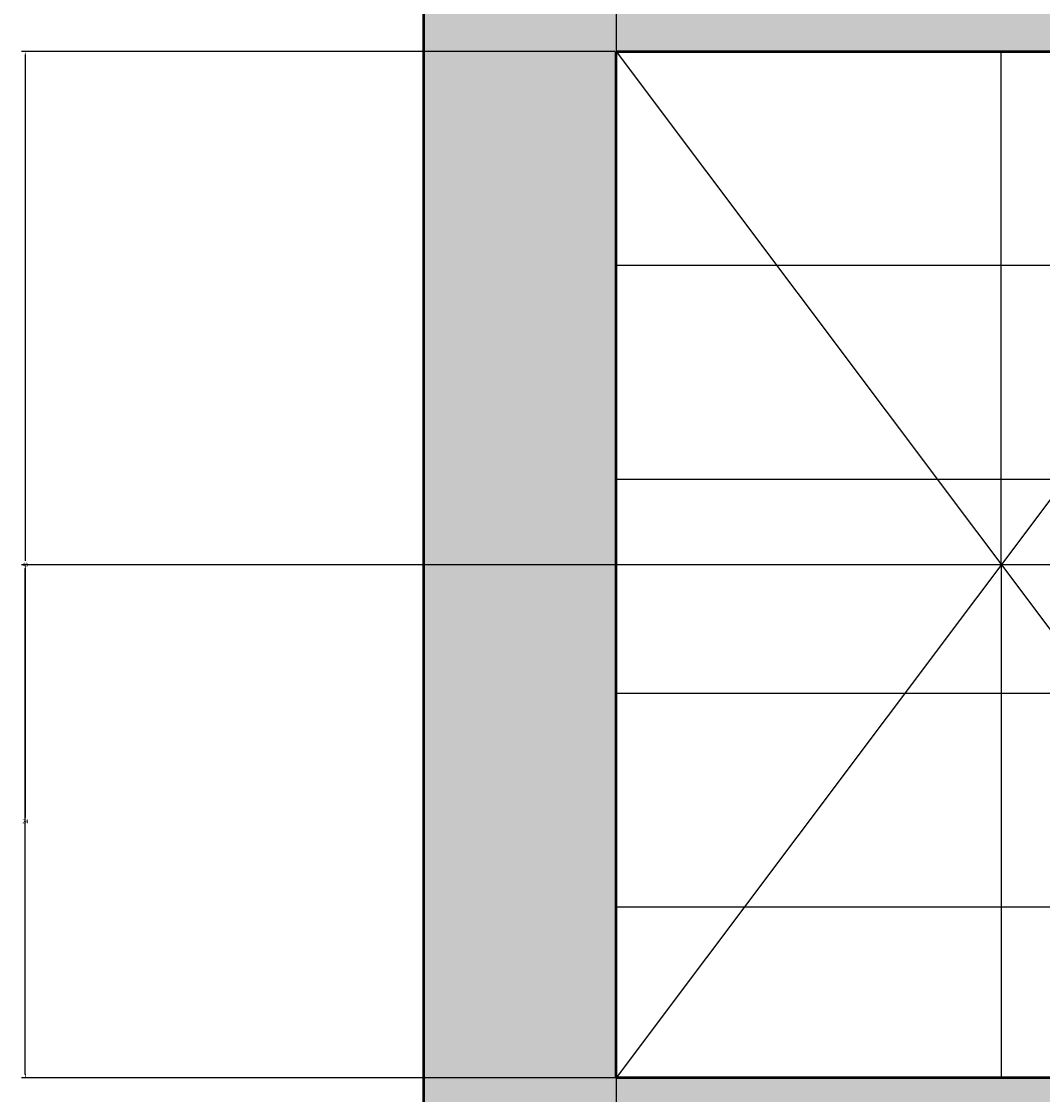
# Model space of a CAD drawing. Units: inches. Extents: x 2231 to 2461, y 2045 to 2455.
# Tile 2 of 95: x 2231 to 2279, y 2072 to 2122. Entities that reach past the tile are written whole.
import ezdxf

# ---------------------------------------------------------------- set-up
doc = ezdxf.new("R2010")
doc.units = ezdxf.units.IN
for name, color, linetype, lineweight in [('A-ANNO-DIMS', 2, 'Continuous', 18), ('A-FLOR-EVTR', 8, 'Continuous', 25), ('A-WALL', 7, 'Continuous', 50)]:
    doc.layers.add(name, color=color, linetype=linetype, lineweight=lineweight)
doc.layers.add('A-WALL-PATT', color=18, linetype='Continuous', lineweight=13, true_color=0x000000)
doc.styles.get("Standard").update_dxf_attribs({"font": 'arial.ttf'})
doc.dimstyles.get("Standard").update_dxf_attribs({"dimtxt": 0.18, "dimasz": 0.18, "dimexe": 0.18, "dimexo": 0.0625, "dimgap": 0.09, "dimtad": 0, "dimtih": 1, "dimtoh": 1, "dimdec": 4, "dimzin": 0, "dimdsep": 46, "dimtxsty": 'Standard', "dimcen": 0.09, "dimadec": 0, "dimazin": 0, "dimtfac": 1, "dimtdec": 4, "dimtofl": 0, "dimtmove": 0, "dimatfit": 3, "dimfxl": 1, "dimtolj": 1, "dimtzin": 0, "dimarcsym": 0})

# ---------------------------------------------------------------- blocks, each defined once
blk = doc.blocks.new('*D51')
at = {"layer": 'A-ANNO-DIMS', "color": 0, "lineweight": -2, "transparency": 16777216}
for p, q in [((2258.794, 2306.77), (2258.794, 2044.803)), ((2330.794, 2306.77), (2330.794, 2044.803)), ((2258.974, 2044.983), (2294.576, 2044.983)), ((2330.614, 2044.983), (2295.011, 2044.983))]:
    blk.add_line(p, q, dxfattribs=at)
at = {"layer": 'A-ANNO-DIMS', "color": 0, "transparency": 16777216}
for points in [[(2258.974, 2045.013), (2258.974, 2044.953), (2258.794, 2044.983)], [(2330.614, 2045.013), (2330.614, 2044.953), (2330.794, 2044.983)]]:
    blk.add_solid(points, dxfattribs=at)
at = {"layer": 'Defpoints', "color": 0, "transparency": 16777216}
for p in [(2258.794, 2306.833), (2330.794, 2306.833), (2330.794, 2044.983)]:
    blk.add_point(p, dxfattribs=at)
at = {"layer": 'A-ANNO-DIMS', "color": 0, "transparency": 16777216, "insert": (2294.794, 2044.983), "char_height": 0.18, "attachment_point": 5}
blk.add_mtext('\\A1;72', dxfattribs=at)
blk = doc.blocks.new('*D61')
at = {"layer": 'A-ANNO-DIMS', "color": 0, "lineweight": -2, "transparency": 16777216}
for p, q in [((2258.731, 2120.833), (2230.981, 2120.833)), ((2231.161, 2120.653), (2231.161, 2097.015)), ((2231.161, 2073.013), (2231.161, 2096.651)), ((2258.731, 2072.833), (2230.981, 2072.833))]:
    blk.add_line(p, q, dxfattribs=at)
at = {"layer": 'A-ANNO-DIMS', "color": 0, "transparency": 16777216}
for points in [[(2231.131, 2120.653), (2231.191, 2120.653), (2231.161, 2120.833)], [(2231.131, 2073.013), (2231.191, 2073.013), (2231.161, 2072.833)]]:
    blk.add_solid(points, dxfattribs=at)
at = {"layer": 'Defpoints', "color": 0, "transparency": 16777216}
for p in [(2231.161, 2120.833), (2258.794, 2120.833), (2258.794, 2072.833)]:
    blk.add_point(p, dxfattribs=at)
at = {"layer": 'A-ANNO-DIMS', "color": 0, "transparency": 16777216, "insert": (2231.161, 2096.833), "char_height": 0.18, "attachment_point": 5}
blk.add_mtext('\\A1;48', dxfattribs=at)
blk = doc.blocks.new('*D67')
at = {"layer": 'A-ANNO-DIMS', "color": 0, "lineweight": -2, "transparency": 16777216}
for p, q in [((2348.126, 2096.833), (2230.981, 2096.833)), ((2231.161, 2096.653), (2231.161, 2085.013)), ((2231.161, 2073.013), (2231.161, 2084.652)), ((2348.559, 2072.833), (2230.981, 2072.833))]:
    blk.add_line(p, q, dxfattribs=at)
at = {"layer": 'A-ANNO-DIMS', "color": 0, "transparency": 16777216}
for points in [[(2231.131, 2096.653), (2231.191, 2096.653), (2231.161, 2096.833)], [(2231.131, 2073.013), (2231.191, 2073.013), (2231.161, 2072.833)]]:
    blk.add_solid(points, dxfattribs=at)
at = {"layer": 'Defpoints', "color": 0, "transparency": 16777216}
for p in [(2348.189, 2096.833), (2231.161, 2072.833), (2348.622, 2072.833)]:
    blk.add_point(p, dxfattribs=at)
at = {"layer": 'A-ANNO-DIMS', "color": 0, "transparency": 16777216, "insert": (2231.161, 2084.833), "char_height": 0.18, "attachment_point": 5}
blk.add_mtext('\\A1;24', dxfattribs=at)

msp = doc.modelspace()

# ---------------------------------------------------------------- hatches: boundary and pattern name
at = {"layer": 'A-WALL-PATT'}
h = msp.add_hatch(color=256, dxfattribs=at)
h.dxf.hatch_style = 1
h.paths.add_polyline_path([(2441.7935, 2269.1535), (2432.7935, 2269.1535), (2432.7935, 2186.8328), (2396.7935, 2186.8328), (2396.7935, 2286.8328), (2394.7935, 2286.8328), (2394.7935, 2186.8328), (2334.7935, 2186.8328), (2334.7935, 2182.8328), (2432.7935, 2182.8328), (2432.7935, 2072.8328), (2416.6639, 2072.8328), (2416.6639, 2063.8328), (2441.7935, 2063.8328)])
h.paths.add_polyline_path([(2368.6639, 2072.8328), (2367.04, 2072.8328), (2330.7942, 2072.8328), (2330.7397, 2063.8328), (2368.6639, 2063.8328)])
h.paths.add_polyline_path([(2300.7392, 2068.3328), (2300.7392, 2072.8328), (2298.7935, 2072.8328), (2294.7935, 2072.8328), (2258.7935, 2072.8328), (2258.7935, 2120.8328), (2294.7935, 2120.8328), (2298.7935, 2120.8328), (2298.7935, 2128.8328), (2294.7935, 2128.8328), (2294.7935, 2124.8328), (2258.7935, 2124.8328), (2258.7935, 2182.8328), (2294.7935, 2182.8328), (2294.7935, 2174.8328), (2298.7935, 2174.8328), (2298.7935, 2182.8328), (2304.7935, 2182.8328), (2304.7935, 2186.8328), (2258.7935, 2186.8328), (2258.7935, 2221.999), (2249.7935, 2221.999), (2249.7935, 2063.8328), (2300.7392, 2063.8328)])
h.paths.add_polyline_path([(2391.9338, 2435.8328), (2333.82, 2435.8328), (2333.82, 2426.8328), (2368.7935, 2426.8328), (2368.7935, 2374.9508), (2368.7935, 2370.8328), (2372.3935, 2370.8328), (2372.7935, 2370.8328), (2372.7935, 2426.8328), (2391.9338, 2426.8328)])
h.paths.add_polyline_path([(2441.7935, 2435.8328), (2415.9338, 2435.8328), (2415.9338, 2426.8328), (2432.7935, 2426.8328), (2432.7935, 2334.8328), (2372.7935, 2334.8328), (2372.7935, 2346.8328), (2368.7935, 2346.8328), (2368.7935, 2306.8328), (2360.7935, 2306.8328), (2360.7935, 2302.8328), (2368.7935, 2302.8328), (2372.7935, 2302.8328), (2372.7935, 2330.8328), (2432.7935, 2330.8328), (2432.7935, 2317.1535), (2441.7935, 2317.1535)])
h.paths.add_polyline_path([(2285.82, 2435.8328), (2249.7935, 2435.8328), (2249.7935, 2269.999), (2258.7935, 2269.999), (2258.7935, 2302.8328), (2318.8168, 2302.8328), (2330.7935, 2302.8328), (2330.7935, 2306.8328), (2258.7935, 2306.8328), (2258.7935, 2426.8328), (2285.82, 2426.8328)])

# ---------------------------------------------------------------- linework, layer by layer
at = {"layer": 'A-FLOR-EVTR'}
for p, q in [((2258.7935, 2120.8328), (2294.7935, 2120.8328)), ((2258.7935, 2072.8328), (2258.7935, 2120.8328)), ((2258.7935, 2120.8328), (2294.7935, 2072.8328)), ((2294.7935, 2120.8328), (2258.7935, 2072.8328)), ((2276.7935, 2096.8328), (2276.7935, 2120.8328)), ((2258.7935, 2110.8328), (2294.7935, 2110.8328)), ((2258.7935, 2100.8328), (2294.7935, 2100.8328)), ((2276.7935, 2096.8328), (2276.7935, 2072.8328)), ((2258.7935, 2090.8328), (2294.7935, 2090.8328)), ((2258.7935, 2080.8328), (2294.7935, 2080.8328)), ((2294.7935, 2072.8328), (2258.7935, 2072.8328))]:
    msp.add_line(p, q, dxfattribs=at)
at = {"layer": 'A-WALL'}
for p, q in [((2258.7935, 2072.8328), (2258.7935, 2120.8328)), ((2258.7935, 2120.8328), (2294.7935, 2120.8328)), ((2294.7935, 2072.8328), (2258.7935, 2072.8328))]:
    msp.add_line(p, q, dxfattribs=at)
msp.add_lwpolyline([(2300.7392, 2063.8328), (2249.7935, 2063.8328), (2249.7935, 2435.8328), (2441.7935, 2435.8328), (2441.7935, 2063.8328), (2330.7397, 2063.8328)], dxfattribs=at)

# ---------------------------------------------------------------- dimensions: what is measured, and where the dimension line sits
at = {"layer": 'A-ANNO-DIMS'}
dim = msp.add_linear_dim(base=(2330.7935, 2044.9825), p1=(2258.7935, 2306.8328), p2=(2330.7935, 2306.8328), dimstyle='Standard', override={"dimdec": 0, "dimlfac": 1, "dimrnd": 0, "dimzin": 0, "dimdsep": 46, "dimlunit": 2}, dxfattribs=at)
dim.commit()
dim.dimension.update_dxf_attribs({"geometry": '*D51', "text_midpoint": (2294.7935, 2044.9825)})
for base, p1, p2, picture, middle in [((2231.161, 2120.8328), (2258.7935, 2072.8328), (2258.7935, 2120.8328), '*D61', (2231.161, 2096.8328)), ((2231.161, 2072.8328), (2348.1888, 2096.8328), (2348.6219, 2072.8328), '*D67', (2231.161, 2084.8328))]:
    dim = msp.add_linear_dim(base=base, p1=p1, p2=p2, angle=90, dimstyle='Standard', override={"dimdec": 0, "dimlfac": 1, "dimrnd": 0, "dimzin": 0, "dimdsep": 46, "dimlunit": 2}, dxfattribs=at)
    dim.commit()
    dim.dimension.update_dxf_attribs({"geometry": picture, "text_midpoint": middle})

doc.saveas('drawing.dxf')
